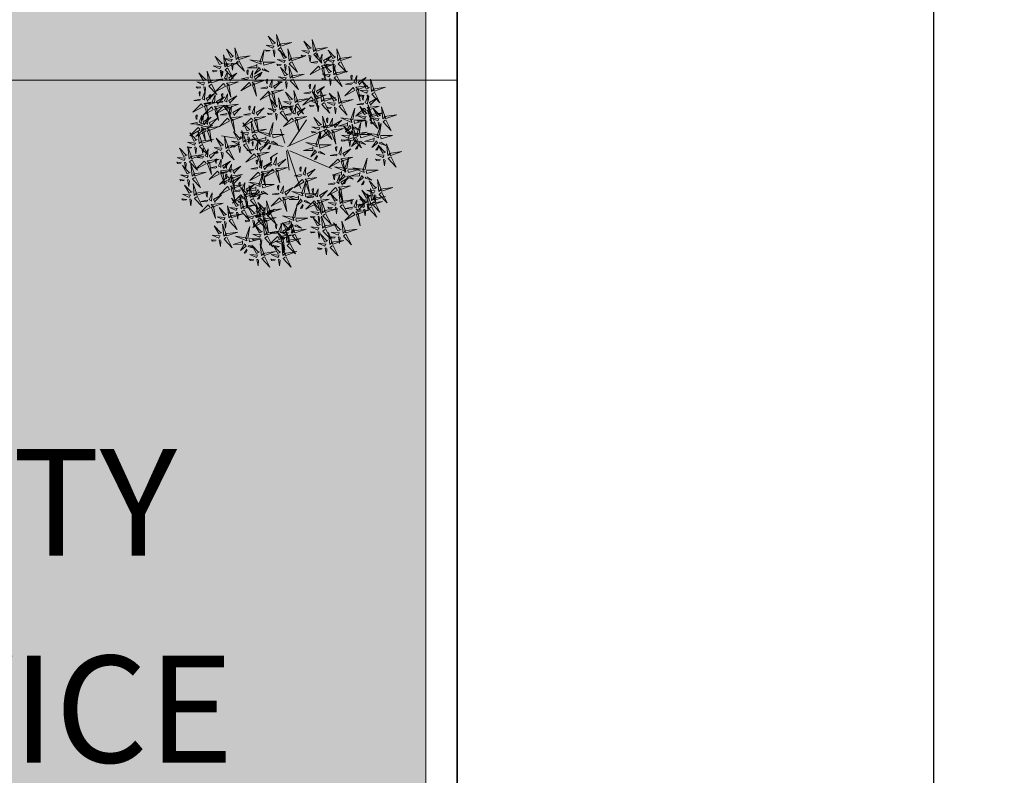
# Model space of a CAD drawing. Units: inches. Extents: x 1704 to 6393, y -157 to 1172.
# Tile 91 of 122: x 2667 to 2793, y 783 to 880. Entities that reach past the tile are written whole.
import ezdxf

# ---------------------------------------------------------------- set-up
doc = ezdxf.new("R2010")
doc.units = ezdxf.units.IN
doc.header["$MEASUREMENT"] = 0
for name, color, linetype, lineweight in [('A-ANNO-DIMS', 7, 'Continuous', 13), ('A-AREA-IDEN', 7, 'Continuous', 18), ('C-PROP', 7, 'Continuous', 35), ('L-HRDS', 8, 'Continuous', 18), ('L-shrub', 74, 'Continuous', 18), ('L-tree', 102, 'Continuous', 18)]:
    doc.layers.add(name, color=color, linetype=linetype, lineweight=lineweight)
doc.layers.add('L-HRDS-PATT', color=9, linetype='Continuous', lineweight=13, true_color=0xc5c1ba)
doc.styles.get("Standard").update_dxf_attribs({"font": 'arial.ttf'})
doc.dimstyles.get("Standard").update_dxf_attribs({"dimtxt": 6, "dimasz": 2, "dimexe": 0.18, "dimexo": 0.0625, "dimgap": 0.09, "dimtad": 0, "dimtih": 1, "dimtoh": 1, "dimdec": 1, "dimzin": 0, "dimdsep": 46, "dimlunit": 3, "dimtxsty": 'Standard', "dimblk": 'ARCHTICK', "dimcen": 0.09, "dimadec": 0, "dimazin": 0, "dimtfac": 1, "dimtdec": 1, "dimtofl": 0, "dimtmove": 0, "dimatfit": 3, "dimfxl": 1, "dimtolj": 1, "dimtzin": 0, "dimarcsym": 0})

# ---------------------------------------------------------------- blocks, each defined once
blk = doc.blocks.new('bamboo')
blk.add_line((390, 162), (546, 218))
at = {"layer": 'L-shrub'}
for p, q in [((-12, 40), (-247, 564)), ((43, 73), (278, 631)), ((-24, 62), (-370, 296)), ((32, 40), (390, 162)), ((-57, 6), (-247, -50)), ((43, 28), (301, 62)), ((-12, -16), (-113, -440)), ((77, -94), (122, -173)), ((-471, -139), (-761, -217)), ((-124, -653), (-158, -842))]:
    blk.add_line(p, q, dxfattribs=at)
for points in [[(-388, 1357), (-437, 1504), (-414, 1335), (-388, 1357)], [(104, 1425), (54, 1572), (78, 1403), (104, 1425)], [(119, 1423), (261, 1497), (148, 1389), (127, 1415)], [(582, 1302), (532, 1450), (556, 1281), (582, 1302)], [(-756, 1207), (-806, 1354), (-782, 1185), (-756, 1207)], [(-412, 1351), (-384, 1316), (-544, 1300), (-421, 1344)], [(-415, 1179), (-464, 1327), (-441, 1158), (-415, 1179)], [(-372, 1355), (-230, 1429), (-344, 1320), (-365, 1346)], [(-161, 1285), (-160, 1445), (-117, 1294), (-150, 1287)], [(-71, 1292), (-28, 1359), (-55, 1273), (-69, 1281)], [(79, 1419), (108, 1385), (-52, 1368), (71, 1412)], [(58, 1358), (77, 1316), (-31, 1255), (65, 1349)], [(103, 1337), (93, 1227), (133, 1319), (110, 1329)], [(168, 1347), (246, 1339), (158, 1324), (159, 1340)], [(597, 1300), (739, 1374), (626, 1266), (604, 1292)], [(704, 1207), (655, 1354), (679, 1185), (704, 1207)], [(-781, 1201), (-752, 1166), (-913, 1150), (-789, 1194)], [(-741, 1205), (-599, 1279), (-712, 1170), (-734, 1196)], [(-562, 1158), (-603, 1137), (-666, 1245), (-570, 1151)], [(-500, 1137), (-534, 1108), (-554, 1268), (-507, 1146)], [(-434, 1290), (-414, 1248), (-523, 1187), (-427, 1281)], [(-388, 1269), (-399, 1159), (-358, 1250), (-381, 1261)], [(-399, 1178), (-257, 1251), (-371, 1143), (-392, 1169)], [(-330, 1216), (-336, 1153), (-319, 1167), (-323, 1207)], [(-324, 1279), (-245, 1271), (-334, 1256), (-332, 1272)], [(-169, 1272), (-323, 1296), (-162, 1239), (-169, 1272)], [(-176, 1248), (-132, 1257), (-192, 1107), (-173, 1237)], [(-131, 1200), (-85, 1198), (-82, 1073), (-120, 1202)], [(-92, 1231), (0, 1171), (-62, 1249), (-81, 1233)], [(-18, 1258), (35, 1223), (30, 1245), (-7, 1260)], [(162, 1284), (156, 1221), (173, 1235), (169, 1276)], [(304, 1094), (304, 1254), (347, 1103), (314, 1096)], [(557, 1296), (586, 1262), (425, 1246), (549, 1289)], [(536, 1235), (555, 1193), (446, 1133), (543, 1226)], [(680, 1201), (709, 1166), (548, 1150), (671, 1194)], [(581, 1215), (571, 1105), (611, 1196), (588, 1206)], [(646, 1224), (724, 1217), (635, 1202), (637, 1217)], [(720, 1205), (862, 1279), (749, 1170), (727, 1196)], [(773, 1166), (723, 1313), (747, 1144), (773, 1166)], [(788, 1164), (930, 1238), (817, 1130), (796, 1155)], [(-835, 1008), (-876, 987), (-939, 1095), (-843, 1001)], [(-802, 1140), (-783, 1098), (-892, 1037), (-795, 1131)], [(-773, 987), (-807, 958), (-827, 1118), (-780, 996)], [(-757, 1119), (-767, 1009), (-727, 1100), (-750, 1111)], [(-698, 1066), (-704, 1003), (-687, 1017), (-691, 1057)], [(-692, 1129), (-614, 1121), (-703, 1106), (-701, 1122)], [(-633, 1052), (-696, 1057), (-682, 1040), (-642, 1045)], [(-581, 1112), (-692, 1120), (-599, 1081), (-590, 1104)], [(-570, 1048), (-576, 969), (-593, 1057), (-578, 1056)], [(-439, 1174), (-411, 1139), (-571, 1123), (-448, 1167)], [(-461, 1112), (-441, 1071), (-550, 1010), (-454, 1104)], [(-495, 1097), (-419, 957), (-529, 1068), (-504, 1090)], [(-494, 1113), (-347, 1165), (-516, 1138), (-494, 1113)], [(-415, 1092), (-426, 982), (-386, 1073), (-408, 1083)], [(-365, 930), (-365, 1090), (-322, 940), (-355, 933)], [(-351, 1102), (-272, 1094), (-361, 1079), (-360, 1095)], [(-156, 961), (-205, 1109), (-182, 940), (-156, 961)], [(-174, 1012), (-174, 1172), (-131, 1021), (-163, 1015)], [(-85, 1020), (-41, 1086), (-69, 1000), (-82, 1009)], [(295, 1081), (141, 1106), (302, 1048), (295, 1081)], [(289, 1057), (332, 1066), (272, 916), (291, 1046)], [(372, 1040), (465, 980), (402, 1058), (383, 1042)], [(393, 1102), (437, 1168), (409, 1082), (396, 1091)], [(446, 1067), (499, 1033), (495, 1054), (457, 1069)], [(658, 1140), (678, 1098), (569, 1037), (665, 1131)], [(748, 1160), (777, 1126), (617, 1109), (740, 1153)], [(640, 1161), (634, 1099), (651, 1113), (647, 1153)], [(727, 1099), (746, 1057), (638, 996), (734, 1090)], [(704, 1119), (694, 1009), (734, 1100), (711, 1111)], [(831, 1008), (789, 987), (726, 1095), (822, 1001)], [(762, 1066), (756, 1003), (774, 1017), (770, 1057)], [(768, 1129), (847, 1121), (758, 1106), (760, 1122)], [(772, 1078), (762, 968), (802, 1060), (779, 1070)], [(837, 1088), (915, 1080), (827, 1065), (828, 1081)], [(892, 987), (859, 958), (839, 1118), (885, 996)], [(-854, 962), (-965, 970), (-872, 931), (-863, 954)], [(-768, 947), (-692, 807), (-802, 918), (-777, 940)], [(-767, 963), (-621, 1015), (-789, 988), (-767, 963)], [(-374, 917), (-528, 942), (-367, 884), (-374, 917)], [(-357, 1039), (-363, 976), (-346, 990), (-350, 1030)], [(-183, 999), (-337, 1024), (-176, 966), (-183, 999)], [(-180, 955), (-152, 921), (-312, 905), (-189, 948)], [(-276, 938), (-232, 1004), (-260, 918), (-273, 927)], [(-189, 975), (-146, 984), (-206, 835), (-187, 964)], [(-145, 927), (-99, 925), (-96, 801), (-134, 929)], [(-140, 960), (2, 1033), (-112, 925), (-133, 951)], [(-106, 958), (-13, 898), (-75, 976), (-95, 960)], [(-32, 985), (21, 951), (17, 973), (-21, 987)], [(290, 849), (291, 1008), (334, 858), (301, 851)], [(333, 1009), (379, 1007), (382, 882), (344, 1011)], [(380, 856), (423, 922), (395, 837), (382, 845)], [(745, 784), (696, 931), (720, 762), (745, 784)], [(811, 962), (701, 970), (793, 931), (803, 954)], [(831, 1025), (825, 962), (842, 976), (838, 1016)], [(897, 947), (974, 807), (863, 918), (889, 940)], [(899, 963), (1045, 1015), (877, 988), (899, 963)], [(1141, 825), (1092, 972), (1115, 803), (1141, 825)], [(-1166, 757), (-1215, 904), (-1192, 735), (-1166, 757)], [(-1150, 755), (-1008, 829), (-1122, 721), (-1143, 746)], [(-975, 702), (-1024, 850), (-1001, 681), (-975, 702)], [(-906, 902), (-969, 907), (-955, 890), (-915, 895)], [(-843, 898), (-849, 819), (-866, 907), (-851, 906)], [(-593, 770), (-642, 918), (-618, 749), (-593, 770)], [(-577, 769), (-435, 842), (-548, 734), (-570, 760)], [(-380, 893), (-337, 902), (-397, 753), (-378, 882)], [(-336, 845), (-290, 844), (-287, 719), (-325, 848)], [(-297, 876), (-204, 816), (-266, 894), (-286, 879)], [(-202, 894), (-182, 853), (-291, 792), (-195, 885)], [(-200, 660), (-234, 631), (-253, 791), (-207, 669)], [(-223, 903), (-170, 869), (-174, 891), (-212, 906)], [(-156, 874), (-167, 764), (-126, 855), (-149, 865)], [(-98, 821), (-104, 758), (-86, 772), (-91, 812)], [(-92, 883), (-13, 876), (-102, 861), (-100, 876)], [(121, 803), (80, 783), (16, 890), (112, 796)], [(281, 835), (128, 860), (288, 803), (281, 835)], [(183, 783), (149, 754), (129, 914), (175, 791)], [(189, 759), (335, 811), (167, 784), (189, 759)], [(275, 811), (319, 820), (259, 671), (277, 800)], [(358, 795), (451, 734), (389, 812), (369, 797)], [(503, 776), (462, 755), (399, 863), (495, 769)], [(433, 822), (486, 787), (481, 809), (444, 824)], [(565, 756), (531, 726), (511, 886), (558, 764)], [(759, 902), (696, 907), (711, 890), (751, 895)], [(761, 782), (903, 856), (790, 748), (768, 774)], [(822, 898), (816, 819), (799, 907), (815, 906)], [(1117, 819), (1145, 785), (985, 768), (1108, 812)], [(1157, 823), (1299, 897), (1185, 789), (1164, 815)], [(1292, 647), (1242, 795), (1266, 626), (1292, 647)], [(-1190, 751), (-1162, 716), (-1322, 700), (-1199, 744)], [(-1212, 690), (-1192, 648), (-1301, 587), (-1205, 681)], [(-1166, 669), (-1177, 559), (-1136, 651), (-1159, 661)], [(-999, 696), (-971, 662), (-1131, 646), (-1008, 689)], [(-1102, 679), (-1023, 671), (-1112, 656), (-1111, 672)], [(-959, 700), (-817, 774), (-931, 666), (-952, 692)], [(-617, 765), (-588, 730), (-749, 714), (-626, 757)], [(-639, 703), (-619, 662), (-728, 601), (-632, 695)], [(-620, 538), (-669, 686), (-646, 517), (-620, 538)], [(-593, 683), (-603, 573), (-563, 664), (-586, 674)], [(-529, 693), (-450, 685), (-539, 670), (-537, 685)], [(-262, 681), (-303, 660), (-366, 768), (-270, 673)], [(-265, 566), (-314, 713), (-291, 544), (-265, 566)], [(-194, 636), (-47, 688), (-216, 661), (-194, 636)], [(49, 698), (-14, 702), (1, 686), (41, 690)], [(101, 757), (-9, 765), (83, 727), (93, 750)], [(112, 693), (106, 614), (89, 703), (105, 701)], [(187, 743), (264, 602), (153, 714), (179, 736)], [(319, 763), (365, 762), (369, 637), (330, 766)], [(432, 670), (369, 675), (383, 658), (423, 663)], [(484, 730), (373, 738), (465, 700), (475, 723)], [(495, 666), (489, 587), (472, 675), (487, 674)], [(570, 716), (646, 575), (536, 686), (561, 708)], [(571, 731), (717, 784), (549, 757), (571, 731)], [(721, 778), (750, 744), (589, 727), (712, 771)], [(699, 717), (719, 675), (610, 614), (706, 708)], [(745, 697), (734, 586), (775, 678), (752, 688)], [(809, 706), (888, 699), (799, 683), (801, 699)], [(868, 552), (819, 700), (842, 531), (868, 552)], [(1095, 758), (1115, 716), (1006, 655), (1102, 749)], [(1073, 552), (1024, 700), (1047, 531), (1073, 552)], [(1141, 737), (1130, 627), (1171, 719), (1148, 729)], [(1199, 684), (1193, 621), (1211, 636), (1206, 676)], [(1205, 747), (1284, 739), (1195, 724), (1197, 740)], [(1307, 646), (1449, 719), (1336, 611), (1314, 637)], [(-1289, 429), (-1338, 577), (-1315, 408), (-1289, 429)], [(-1122, 544), (-1163, 524), (-1226, 631), (-1130, 537)], [(-1108, 616), (-1114, 553), (-1097, 567), (-1101, 607)], [(-1060, 524), (-1094, 495), (-1113, 654), (-1067, 532)], [(-1021, 635), (-1001, 593), (-1110, 533), (-1014, 626)], [(-1054, 499), (-907, 552), (-1076, 525), (-1054, 499)], [(-975, 615), (-986, 505), (-945, 596), (-968, 606)], [(-917, 561), (-923, 499), (-906, 513), (-910, 553)], [(-911, 624), (-832, 617), (-921, 602), (-919, 617)], [(-712, 449), (-753, 428), (-816, 536), (-721, 441)], [(-644, 533), (-616, 498), (-776, 482), (-653, 526)], [(-650, 428), (-684, 399), (-704, 559), (-658, 437)], [(-604, 537), (-462, 610), (-576, 502), (-597, 528)], [(-535, 630), (-541, 567), (-523, 581), (-527, 621)], [(-289, 560), (-261, 526), (-421, 509), (-298, 553)], [(-333, 575), (-396, 580), (-381, 563), (-341, 568)], [(-281, 634), (-391, 643), (-299, 604), (-289, 627)], [(-270, 570), (-276, 492), (-293, 580), (-277, 579)], [(-249, 564), (-107, 638), (-221, 530), (-242, 555)], [(-195, 620), (-118, 480), (-229, 591), (-203, 613)], [(-38, 467), (-37, 627), (6, 476), (-27, 469)], [(52, 474), (95, 540), (68, 455), (54, 463)], [(680, 490), (639, 469), (576, 577), (672, 482)], [(742, 469), (708, 440), (689, 600), (735, 478)], [(844, 546), (872, 512), (712, 496), (835, 539)], [(803, 643), (797, 580), (815, 595), (810, 635)], [(884, 550), (1026, 624), (912, 516), (891, 542)], [(1049, 546), (1077, 512), (917, 496), (1040, 539)], [(1089, 550), (1231, 624), (1117, 516), (1096, 542)], [(1267, 642), (1296, 607), (1135, 591), (1259, 635)], [(1245, 580), (1265, 539), (1156, 478), (1253, 572)], [(1291, 560), (1281, 450), (1321, 541), (1298, 552)], [(1356, 570), (1434, 562), (1345, 547), (1347, 563)], [(-1313, 424), (-1285, 389), (-1445, 373), (-1322, 417)], [(-1273, 428), (-1131, 501), (-1245, 393), (-1266, 419)], [(-1193, 439), (-1256, 443), (-1242, 426), (-1202, 431)], [(-1141, 498), (-1251, 506), (-1159, 468), (-1150, 491)], [(-1130, 434), (-1136, 355), (-1153, 444), (-1137, 442)], [(-1055, 484), (-979, 343), (-1089, 455), (-1063, 476)], [(-731, 403), (-842, 411), (-750, 372), (-740, 395)], [(-666, 471), (-646, 430), (-755, 369), (-659, 463)], [(-644, 404), (-498, 456), (-666, 429), (-644, 404)], [(-620, 451), (-631, 341), (-590, 432), (-613, 442)], [(-562, 398), (-568, 335), (-551, 349), (-555, 389)], [(-556, 461), (-477, 453), (-566, 438), (-564, 454)], [(-311, 499), (-291, 457), (-400, 396), (-304, 490)], [(-265, 478), (-276, 368), (-235, 460), (-258, 470)], [(-207, 425), (-213, 362), (-196, 376), (-200, 416)], [(-201, 488), (-122, 480), (-211, 465), (-210, 481)], [(-46, 454), (-200, 478), (-40, 421), (-46, 454)], [(-53, 429), (-9, 439), (-69, 289), (-50, 418)], [(31, 413), (123, 352), (61, 431), (42, 415)], [(105, 440), (158, 405), (153, 427), (116, 442)], [(394, 326), (353, 305), (290, 413), (385, 319)], [(456, 306), (422, 276), (402, 436), (448, 314)], [(661, 444), (551, 452), (643, 413), (653, 436)], [(618, 276), (618, 436), (661, 285), (628, 278)], [(747, 429), (824, 289), (713, 400), (739, 422)], [(748, 445), (895, 497), (727, 470), (748, 445)], [(822, 485), (842, 443), (733, 383), (829, 476)], [(868, 465), (857, 355), (898, 446), (875, 456)], [(926, 411), (920, 349), (937, 363), (933, 403)], [(932, 474), (1011, 467), (922, 452), (924, 467)], [(1027, 485), (1047, 443), (938, 383), (1034, 476)], [(1073, 465), (1062, 355), (1103, 446), (1080, 456)], [(1131, 411), (1125, 349), (1142, 363), (1138, 403)], [(1137, 474), (1216, 467), (1127, 452), (1128, 467)], [(1349, 507), (1343, 444), (1361, 458), (1357, 498)], [(-1335, 362), (-1315, 321), (-1424, 260), (-1328, 354)], [(-1289, 342), (-1300, 232), (-1259, 323), (-1282, 333)], [(-1231, 289), (-1237, 226), (-1220, 240), (-1224, 280)], [(-1225, 352), (-1146, 344), (-1235, 329), (-1233, 345)], [(-784, 343), (-847, 348), (-832, 331), (-792, 336)], [(-721, 338), (-727, 260), (-744, 348), (-728, 347)], [(-645, 388), (-569, 248), (-679, 359), (-654, 381)], [(-606, 184), (-656, 331), (-632, 163), (-606, 184)], [(-425, 190), (-467, 169), (-530, 277), (-434, 182)], [(-364, 169), (-397, 140), (-417, 300), (-371, 178)], [(-8, 382), (38, 380), (41, 255), (2, 384)], [(374, 280), (264, 288), (356, 250), (366, 273)], [(460, 266), (537, 125), (427, 236), (452, 258)], [(462, 281), (608, 334), (440, 307), (462, 281)], [(609, 263), (455, 287), (616, 230), (609, 263)], [(609, 384), (546, 389), (561, 372), (601, 377)], [(672, 379), (666, 301), (649, 389), (665, 388)], [(707, 283), (751, 349), (723, 264), (710, 272)], [(945, 153), (946, 313), (989, 162), (956, 155)], [(1141, 143), (1092, 291), (1115, 122), (1141, 143)], [(-1166, 102), (-1215, 250), (-1192, 81), (-1166, 102)], [(-1150, 100), (-1008, 174), (-1122, 66), (-1143, 92)], [(-934, 116), (-983, 263), (-960, 94), (-934, 116)], [(-918, 114), (-776, 188), (-890, 80), (-911, 105)], [(-631, 178), (-602, 144), (-762, 128), (-639, 171)], [(-590, 182), (-449, 256), (-562, 148), (-583, 174)], [(-445, 144), (-555, 152), (-463, 113), (-453, 136)], [(-358, 145), (-211, 197), (-379, 170), (-358, 145)], [(322, 220), (259, 225), (274, 208), (314, 213)], [(385, 216), (379, 137), (362, 225), (378, 224)], [(603, 239), (646, 248), (586, 98), (605, 228)], [(647, 191), (693, 189), (696, 64), (658, 193)], [(701, 6), (667, -24), (648, 136), (694, 14)], [(686, 222), (779, 161), (716, 240), (697, 224)], [(760, 249), (813, 214), (809, 236), (771, 251)], [(937, 140), (783, 165), (943, 107), (937, 140)], [(1117, 137), (1145, 103), (985, 87), (1108, 130)], [(1035, 161), (1078, 227), (1051, 141), (1037, 150)], [(1157, 141), (1299, 215), (1185, 107), (1164, 133)], [(1264, 75), (1215, 222), (1238, 53), (1264, 75)], [(1280, 73), (1422, 147), (1308, 39), (1287, 65)], [(1442, 20), (1392, 168), (1416, -1), (1442, 20)], [(-1357, -48), (-1406, 100), (-1383, -69), (-1357, -48)], [(-1341, -50), (-1199, 24), (-1313, -84), (-1334, -58)], [(-1190, 96), (-1162, 62), (-1322, 46), (-1199, 89)], [(-1212, 35), (-1192, -7), (-1301, -67), (-1205, 26)], [(-1166, 15), (-1177, -95), (-1136, -4), (-1159, 6)], [(-1102, 24), (-1023, 17), (-1112, 2), (-1111, 17)], [(-958, 110), (-930, 76), (-1090, 59), (-967, 103)], [(-980, 49), (-960, 7), (-1069, -54), (-973, 40)], [(-934, 28), (-945, -82), (-904, 10), (-927, 20)], [(-870, 38), (-791, 30), (-880, 15), (-878, 31)], [(-652, 117), (-632, 75), (-741, 14), (-645, 108)], [(-607, 97), (-617, -13), (-577, 78), (-600, 88)], [(-511, -21), (-560, 127), (-536, -42), (-511, -21)], [(-497, 84), (-560, 89), (-545, 72), (-505, 77)], [(-548, 43), (-554, -20), (-537, -5), (-541, 35)], [(-542, 106), (-464, 99), (-552, 83), (-551, 99)], [(-495, -22), (-353, 51), (-466, -57), (-488, -31)], [(-434, 79), (-440, 1), (-457, 89), (-441, 88)], [(-359, 129), (-282, -11), (-393, 100), (-367, 122)], [(257, -69), (216, -90), (153, 18), (249, -77)], [(319, -90), (285, -119), (266, 41), (312, -81)], [(640, 26), (598, 5), (535, 113), (631, 19)], [(707, -19), (854, 34), (686, 7), (707, -19)], [(930, 116), (974, 125), (914, -24), (932, 105)], [(974, 68), (1021, 66), (1024, -58), (985, 70)], [(1095, 76), (1115, 34), (1006, -27), (1102, 67)], [(1014, 99), (1106, 39), (1044, 117), (1025, 101)], [(1158, -1), (1117, -22), (1054, 86), (1150, -9)], [(1088, 126), (1141, 92), (1136, 113), (1099, 128)], [(1240, 69), (1268, 35), (1108, 18), (1231, 62)], [(1218, 8), (1238, -34), (1129, -95), (1225, -1)], [(1141, 56), (1130, -54), (1171, 37), (1148, 47)], [(1220, -22), (1186, -51), (1167, 109), (1213, -13)], [(1199, 2), (1193, -60), (1211, -46), (1206, -6)], [(1205, 65), (1284, 58), (1195, 42), (1197, 58)], [(1226, -46), (1373, 6), (1204, -21), (1226, -46)], [(1417, 15), (1446, -20), (1286, -36), (1409, 8)], [(1457, 19), (1599, 92), (1486, -16), (1465, 10)], [(-1381, -54), (-1353, -88), (-1513, -104), (-1390, -61)], [(-1403, -115), (-1383, -157), (-1492, -217), (-1396, -124)], [(-1293, -126), (-1215, -133), (-1303, -148), (-1302, -133)], [(-1144, -283), (-1143, -123), (-1100, -274), (-1133, -281)], [(-1108, -39), (-1114, -101), (-1097, -87), (-1101, -47)], [(-780, -124), (-822, -145), (-885, -37), (-789, -131)], [(-876, -25), (-882, -88), (-865, -74), (-869, -33)], [(-719, -144), (-752, -174), (-772, -14), (-726, -136)], [(-712, -169), (-566, -116), (-734, -143), (-712, -169)], [(-535, -26), (-507, -61), (-667, -77), (-544, -33)], [(-557, -88), (-537, -129), (-646, -190), (-550, -96)], [(-511, -108), (-522, -218), (-481, -127), (-504, -117)], [(-447, -98), (-368, -106), (-457, -121), (-455, -105)], [(-174, -160), (-174, -1), (-131, -151), (-163, -158)], [(-85, -153), (-41, -87), (-69, -173), (-82, -164)], [(238, -116), (128, -107), (220, -146), (229, -123)], [(324, -130), (400, -270), (290, -159), (315, -137)], [(325, -114), (472, -62), (303, -89), (325, -114)], [(568, -80), (505, -75), (520, -92), (560, -87)], [(620, -20), (510, -12), (602, -50), (612, -27)], [(631, -84), (625, -163), (608, -75), (624, -76)], [(706, -34), (783, -175), (672, -64), (698, -42)], [(868, -184), (819, -37), (842, -206), (868, -184)], [(884, -186), (1026, -112), (912, -220), (891, -194)], [(988, -240), (954, -269), (935, -109), (981, -231)], [(1087, -107), (1024, -102), (1038, -119), (1078, -114)], [(1139, -47), (1029, -39), (1121, -78), (1130, -55)], [(1169, -225), (1119, -78), (1143, -247), (1169, -225)], [(1150, -112), (1144, -190), (1127, -102), (1143, -103)], [(1225, -62), (1301, -202), (1191, -91), (1217, -69)], [(1264, -13), (1253, -123), (1294, -31), (1271, -21)], [(1396, -47), (1415, -88), (1306, -149), (1403, -55)], [(1322, -66), (1316, -129), (1333, -114), (1329, -74)], [(1328, -3), (1407, -10), (1318, -26), (1320, -10)], [(1442, -266), (1392, -119), (1416, -287), (1442, -266)], [(1441, -67), (1431, -177), (1471, -86), (1448, -76)], [(1500, -120), (1494, -183), (1511, -169), (1507, -129)], [(1506, -57), (1584, -65), (1496, -80), (1497, -65)], [(-1358, -135), (-1368, -245), (-1328, -154), (-1350, -144)], [(-1299, -188), (-1305, -251), (-1288, -237), (-1292, -197)], [(-1054, -276), (-1011, -210), (-1038, -295), (-1052, -287)], [(-852, -230), (-915, -225), (-900, -242), (-860, -237)], [(-800, -170), (-910, -162), (-818, -200), (-808, -177)], [(-789, -234), (-795, -313), (-812, -225), (-796, -226)], [(-714, -184), (-637, -325), (-748, -214), (-722, -192)], [(-453, -161), (-459, -224), (-441, -210), (-446, -170)], [(-364, -376), (-397, -405), (-417, -246), (-371, -368)], [(-183, -174), (-337, -149), (-176, -206), (-183, -174)], [(-197, -389), (-246, -241), (-222, -410), (-197, -389)], [(-189, -198), (-146, -189), (-206, -338), (-187, -209)], [(-145, -246), (-99, -247), (-96, -372), (-134, -243)], [(-106, -215), (-13, -275), (-75, -197), (-95, -212)], [(52, -315), (11, -336), (-52, -228), (44, -322)], [(-32, -187), (21, -222), (17, -200), (-21, -185)], [(114, -335), (80, -364), (61, -205), (107, -327)], [(186, -175), (123, -170), (137, -187), (177, -182)], [(298, -260), (257, -281), (194, -173), (290, -268)], [(249, -180), (243, -258), (226, -170), (242, -171)], [(360, -281), (326, -310), (307, -150), (353, -272)], [(366, -305), (513, -253), (344, -280), (366, -305)], [(495, -297), (495, -137), (538, -288), (506, -295)], [(584, -289), (628, -223), (600, -309), (587, -300)], [(844, -190), (872, -224), (712, -241), (835, -197)], [(822, -251), (842, -293), (733, -354), (829, -260)], [(907, -266), (797, -257), (889, -296), (898, -273)], [(926, -219), (885, -240), (822, -132), (918, -227)], [(923, -321), (874, -173), (897, -342), (923, -321)], [(932, -262), (1011, -270), (922, -285), (924, -269)], [(939, -322), (1081, -249), (967, -357), (946, -331)], [(994, -264), (1141, -212), (972, -239), (994, -264)], [(1144, -231), (1173, -265), (1013, -282), (1136, -238)], [(1184, -227), (1326, -153), (1213, -261), (1191, -235)], [(1457, -268), (1599, -194), (1486, -302), (1465, -276)], [(-1152, -296), (-1306, -272), (-1145, -329), (-1152, -296)], [(-1159, -321), (-1115, -311), (-1175, -461), (-1156, -331)], [(-1114, -368), (-1068, -370), (-1065, -495), (-1103, -366)], [(-1075, -337), (-983, -398), (-1045, -319), (-1064, -335)], [(-903, -383), (-944, -404), (-1007, -296), (-912, -390)], [(-1001, -310), (-948, -345), (-953, -323), (-990, -308)], [(-841, -404), (-875, -433), (-895, -273), (-849, -395)], [(-835, -428), (-689, -375), (-857, -402), (-835, -428)], [(-445, -402), (-555, -394), (-463, -432), (-453, -409)], [(-425, -356), (-467, -376), (-530, -269), (-434, -363)], [(-358, -400), (-211, -348), (-379, -375), (-358, -400)], [(-221, -394), (-193, -429), (-353, -445), (-230, -402)], [(-181, -390), (-39, -317), (-152, -425), (-174, -399)], [(-74, -512), (-123, -364), (-100, -533), (-74, -512)], [(33, -361), (-77, -353), (15, -391), (25, -368)], [(119, -375), (196, -516), (85, -404), (111, -383)], [(120, -360), (267, -307), (99, -334), (120, -360)], [(227, -366), (164, -361), (178, -378), (218, -373)], [(279, -306), (169, -298), (261, -337), (270, -314)], [(290, -371), (284, -449), (267, -361), (283, -362)], [(365, -321), (441, -461), (331, -350), (356, -328)], [(486, -310), (332, -285), (493, -343), (486, -310)], [(480, -334), (523, -325), (463, -474), (482, -345)], [(524, -382), (570, -384), (573, -508), (535, -380)], [(563, -351), (656, -411), (594, -333), (574, -349)], [(660, -513), (626, -542), (607, -382), (653, -504)], [(663, -416), (614, -269), (638, -437), (663, -416)], [(637, -324), (690, -358), (686, -336), (648, -322)], [(679, -418), (821, -344), (708, -452), (686, -426)], [(814, -539), (764, -391), (788, -560), (814, -539)], [(899, -326), (927, -361), (767, -377), (890, -333)], [(877, -388), (897, -429), (788, -490), (884, -396)], [(855, -325), (792, -320), (806, -337), (846, -332)], [(868, -272), (857, -382), (898, -290), (875, -280)], [(918, -330), (912, -408), (895, -320), (911, -321)], [(926, -325), (920, -388), (937, -374), (933, -333)], [(993, -280), (1069, -420), (959, -309), (984, -287)], [(1123, -292), (1142, -334), (1033, -395), (1130, -301)], [(1168, -312), (1158, -423), (1198, -331), (1175, -321)], [(1218, -474), (1219, -314), (1262, -465), (1229, -472)], [(1227, -366), (1221, -429), (1238, -414), (1234, -374)], [(1233, -303), (1311, -310), (1223, -326), (1224, -310)], [(1417, -272), (1446, -306), (1286, -322), (1409, -279)], [(1396, -333), (1415, -375), (1306, -436), (1403, -342)], [(1441, -353), (1431, -463), (1471, -372), (1448, -362)], [(1506, -344), (1584, -351), (1496, -367), (1497, -351)], [(-1180, -607), (-1229, -459), (-1205, -628), (-1180, -607)], [(-975, -489), (-1038, -484), (-1023, -501), (-983, -496)], [(-923, -429), (-1033, -421), (-941, -459), (-931, -436)], [(-912, -493), (-918, -572), (-935, -484), (-919, -485)], [(-837, -444), (-760, -584), (-870, -473), (-845, -451)], [(-497, -461), (-560, -457), (-545, -474), (-505, -469)], [(-434, -466), (-440, -545), (-457, -456), (-441, -458)], [(-359, -416), (-282, -557), (-393, -445), (-367, -424)], [(-243, -456), (-223, -497), (-332, -558), (-236, -464)], [(-98, -517), (-70, -552), (-230, -568), (-107, -524)], [(-197, -476), (-208, -586), (-167, -495), (-190, -485)], [(-133, -466), (-54, -474), (-143, -489), (-141, -474)], [(-19, -420), (-82, -416), (-67, -433), (-27, -428)], [(-58, -513), (84, -440), (-30, -548), (-51, -522)], [(44, -425), (38, -504), (21, -415), (37, -417)], [(599, -492), (557, -513), (494, -405), (590, -499)], [(639, -422), (668, -456), (507, -472), (631, -429)], [(617, -483), (637, -525), (528, -586), (625, -492)], [(666, -537), (813, -484), (645, -511), (666, -537)], [(663, -503), (653, -613), (693, -522), (670, -512)], [(727, -494), (806, -501), (717, -517), (719, -501)], [(829, -540), (971, -467), (858, -575), (836, -549)], [(922, -408), (912, -518), (952, -427), (930, -417)], [(981, -461), (975, -524), (992, -510), (988, -470)], [(987, -398), (1065, -406), (977, -421), (978, -405)], [(1210, -487), (1056, -463), (1216, -520), (1210, -487)], [(1203, -511), (1247, -502), (1187, -652), (1206, -522)], [(1287, -528), (1379, -588), (1317, -510), (1298, -526)], [(1308, -467), (1351, -400), (1324, -486), (1310, -478)], [(1361, -501), (1414, -536), (1409, -514), (1372, -499)], [(1500, -407), (1494, -470), (1511, -455), (1507, -415)], [(-1204, -613), (-1176, -647), (-1336, -663), (-1213, -620)], [(-1164, -609), (-1022, -535), (-1135, -643), (-1157, -617)], [(-1084, -757), (-1133, -609), (-1110, -778), (-1084, -757)], [(-890, -724), (-931, -745), (-994, -637), (-898, -731)], [(-828, -744), (-862, -774), (-881, -614), (-835, -736)], [(-589, -724), (-630, -745), (-693, -637), (-598, -731)], [(-527, -744), (-561, -774), (-581, -614), (-535, -736)], [(-425, -669), (-467, -690), (-530, -582), (-434, -677)], [(-364, -690), (-397, -719), (-417, -559), (-371, -681)], [(-120, -579), (-100, -620), (-209, -681), (-113, -587)], [(-139, -529), (-145, -592), (-127, -578), (-132, -538)], [(-74, -599), (-85, -709), (-44, -618), (-67, -607)], [(8, -743), (-41, -596), (-18, -765), (8, -743)], [(-16, -652), (-22, -715), (-5, -701), (-9, -661)], [(-10, -589), (69, -597), (-20, -612), (-18, -596)], [(353, -669), (312, -690), (249, -582), (344, -677)], [(415, -690), (381, -719), (361, -559), (407, -681)], [(489, -669), (448, -690), (385, -582), (481, -677)], [(527, -598), (464, -593), (479, -610), (519, -605)], [(579, -538), (469, -530), (561, -569), (571, -546)], [(551, -690), (517, -719), (498, -559), (544, -681)], [(590, -602), (584, -681), (567, -593), (583, -594)], [(665, -553), (742, -693), (631, -582), (657, -560)], [(789, -544), (818, -579), (658, -595), (781, -552)], [(768, -606), (787, -647), (678, -708), (775, -614)], [(721, -557), (715, -620), (733, -605), (729, -565)], [(813, -626), (803, -736), (843, -645), (820, -635)], [(878, -616), (956, -624), (868, -639), (869, -624)], [(937, -703), (887, -555), (911, -724), (937, -703)], [(952, -704), (1094, -630), (981, -739), (959, -713)], [(1182, -771), (1133, -623), (1156, -792), (1182, -771)], [(1248, -559), (1294, -561), (1297, -686), (1258, -557)], [(-1226, -674), (-1206, -716), (-1315, -776), (-1219, -683)], [(-1108, -763), (-1080, -797), (-1240, -813), (-1117, -770)], [(-1180, -694), (-1191, -804), (-1150, -713), (-1173, -703)], [(-1122, -748), (-1128, -810), (-1110, -796), (-1115, -756)], [(-1116, -685), (-1037, -692), (-1126, -707), (-1124, -692)], [(-1068, -759), (-926, -685), (-1040, -793), (-1061, -767)], [(-909, -770), (-1019, -762), (-927, -800), (-917, -777)], [(-823, -784), (-746, -925), (-857, -814), (-831, -792)], [(-822, -769), (-675, -716), (-844, -743), (-822, -769)], [(-609, -770), (-719, -762), (-627, -800), (-617, -777)], [(-514, -908), (-548, -937), (-567, -777), (-521, -900)], [(-497, -775), (-560, -770), (-545, -787), (-505, -782)], [(-523, -784), (-446, -925), (-556, -814), (-531, -792)], [(-445, -715), (-555, -707), (-463, -746), (-453, -723)], [(-521, -769), (-375, -716), (-543, -743), (-521, -769)], [(-434, -780), (-440, -858), (-457, -770), (-441, -771)], [(-359, -730), (-282, -870), (-393, -759), (-367, -737)], [(-358, -714), (-211, -662), (-379, -689), (-358, -714)], [(-16, -749), (12, -783), (-148, -800), (-25, -756)], [(24, -745), (166, -671), (52, -779), (31, -754)], [(285, -806), (243, -826), (180, -719), (276, -813)], [(281, -775), (218, -770), (233, -787), (273, -782)], [(333, -715), (223, -707), (315, -746), (325, -723)], [(346, -826), (312, -855), (293, -696), (339, -818)], [(344, -780), (338, -858), (321, -770), (337, -771)], [(418, -775), (355, -770), (369, -787), (409, -782)], [(470, -715), (360, -707), (452, -746), (462, -723)], [(419, -730), (496, -870), (386, -759), (411, -737)], [(421, -714), (567, -662), (399, -689), (421, -714)], [(481, -780), (475, -858), (458, -770), (474, -771)], [(556, -730), (632, -870), (522, -759), (548, -737)], [(557, -714), (704, -662), (535, -689), (557, -714)], [(912, -708), (941, -743), (780, -759), (904, -715)], [(890, -769), (910, -811), (801, -872), (898, -778)], [(872, -679), (866, -742), (883, -728), (879, -688)], [(936, -790), (926, -900), (966, -809), (943, -798)], [(1001, -780), (1079, -788), (990, -803), (992, -787)], [(1158, -776), (1186, -811), (1026, -827), (1149, -783)], [(1198, -772), (1340, -699), (1226, -807), (1205, -781)], [(-1130, -824), (-1110, -866), (-1219, -926), (-1123, -833)], [(-1084, -844), (-1095, -954), (-1055, -863), (-1077, -853)], [(-1026, -898), (-1032, -960), (-1015, -946), (-1019, -906)], [(-1020, -835), (-941, -842), (-1030, -857), (-1029, -842)], [(-961, -829), (-1024, -825), (-1009, -842), (-969, -837)], [(-898, -834), (-904, -913), (-921, -825), (-905, -826)], [(-866, -975), (-915, -828), (-891, -997), (-866, -975)], [(-850, -977), (-708, -903), (-821, -1011), (-843, -985)], [(-661, -829), (-724, -825), (-709, -842), (-669, -837)], [(-576, -888), (-617, -908), (-680, -801), (-584, -895)], [(-598, -834), (-604, -913), (-621, -825), (-605, -826)], [(-555, -1044), (-589, -1074), (-608, -914), (-562, -1036)], [(-508, -932), (-361, -880), (-530, -907), (-508, -932)], [(-289, -983), (-330, -1004), (-393, -896), (-297, -990)], [(-227, -1004), (-261, -1033), (-280, -873), (-234, -995)], [(-38, -810), (-18, -852), (-127, -913), (-31, -819)], [(8, -831), (-3, -941), (38, -849), (15, -839)], [(148, -983), (107, -1004), (44, -896), (140, -990)], [(66, -884), (60, -947), (77, -933), (73, -893)], [(72, -821), (151, -829), (62, -844), (64, -828)], [(213, -911), (150, -907), (165, -924), (205, -919)], [(265, -852), (155, -844), (247, -882), (257, -859)], [(210, -1004), (176, -1033), (156, -873), (203, -995)], [(276, -916), (270, -995), (253, -906), (269, -908)], [(351, -866), (428, -1007), (317, -895), (343, -873)], [(352, -850), (499, -798), (331, -825), (352, -850)], [(735, -928), (694, -949), (631, -841), (727, -936)], [(797, -949), (763, -978), (743, -818), (790, -941)], [(803, -973), (950, -921), (781, -948), (803, -973)], [(995, -843), (989, -906), (1006, -892), (1002, -852)], [(1136, -838), (1156, -879), (1047, -940), (1143, -846)], [(1182, -858), (1171, -968), (1212, -877), (1189, -867)], [(1240, -911), (1234, -974), (1251, -960), (1247, -920)], [(1246, -848), (1325, -856), (1236, -871), (1238, -855)], [(-890, -981), (-862, -1015), (-1022, -1032), (-899, -988)], [(-912, -1042), (-892, -1084), (-1001, -1145), (-905, -1051)], [(-802, -1053), (-723, -1060), (-812, -1076), (-810, -1060)], [(-617, -1024), (-658, -1045), (-721, -937), (-625, -1031)], [(-647, -993), (-710, -988), (-695, -1005), (-655, -1000)], [(-595, -934), (-705, -925), (-613, -964), (-603, -941)], [(-584, -998), (-590, -1077), (-607, -988), (-591, -989)], [(-549, -1069), (-402, -1016), (-570, -1043), (-549, -1069)], [(-509, -948), (-432, -1088), (-543, -977), (-517, -955)], [(-308, -1029), (-418, -1021), (-326, -1059), (-317, -1036)], [(-303, -1065), (-344, -1086), (-407, -978), (-311, -1072)], [(-241, -1085), (-275, -1114), (-294, -955), (-248, -1077)], [(-222, -1043), (-146, -1184), (-256, -1073), (-231, -1051)], [(-221, -1028), (-74, -975), (-243, -1002), (-221, -1028)], [(-60, -1098), (-109, -950), (-86, -1119), (-60, -1098)], [(-44, -1099), (98, -1026), (-16, -1134), (-37, -1108)], [(129, -1029), (18, -1021), (111, -1059), (120, -1036)], [(215, -1043), (291, -1184), (181, -1073), (206, -1051)], [(216, -1028), (362, -975), (194, -1002), (216, -1028)], [(377, -1193), (327, -1046), (351, -1215), (377, -1193)], [(636, -1166), (587, -1019), (610, -1187), (636, -1166)], [(664, -1034), (601, -1029), (615, -1046), (655, -1041)], [(716, -975), (605, -966), (698, -1005), (707, -982)], [(727, -1039), (721, -1117), (704, -1029), (719, -1030)], [(802, -989), (878, -1129), (768, -1018), (793, -996)], [(-866, -1062), (-877, -1173), (-836, -1081), (-859, -1071)], [(-808, -1116), (-814, -1179), (-796, -1164), (-801, -1124)], [(-688, -1129), (-751, -1125), (-736, -1142), (-696, -1137)], [(-636, -1070), (-746, -1062), (-654, -1100), (-644, -1077)], [(-625, -1134), (-631, -1213), (-648, -1125), (-632, -1126)], [(-550, -1084), (-473, -1225), (-584, -1114), (-558, -1092)], [(-374, -1170), (-437, -1166), (-422, -1183), (-382, -1178)], [(-322, -1111), (-432, -1103), (-340, -1141), (-330, -1118)], [(-360, -1089), (-423, -1084), (-409, -1101), (-369, -1096)], [(-311, -1175), (-317, -1254), (-334, -1165), (-318, -1167)], [(-297, -1093), (-303, -1172), (-320, -1084), (-305, -1085)], [(-236, -1125), (-159, -1266), (-270, -1154), (-244, -1133)], [(-235, -1110), (-88, -1057), (-256, -1084), (-235, -1110)], [(-84, -1104), (-56, -1138), (-216, -1154), (-93, -1111)], [(-106, -1165), (-86, -1206), (-195, -1267), (-99, -1174)], [(-61, -1185), (-71, -1295), (-31, -1204), (-53, -1194)], [(4, -1176), (83, -1183), (-6, -1198), (-5, -1183)], [(77, -1089), (14, -1084), (28, -1101), (68, -1096)], [(145, -1234), (95, -1087), (119, -1256), (145, -1234)], [(140, -1093), (134, -1172), (117, -1084), (132, -1085)], [(160, -1236), (302, -1162), (189, -1270), (168, -1244)], [(393, -1195), (534, -1121), (421, -1229), (400, -1204)], [(612, -1172), (640, -1206), (480, -1222), (603, -1179)], [(652, -1168), (794, -1094), (680, -1202), (659, -1176)], [(120, -1240), (149, -1274), (-11, -1291), (112, -1247)], [(-2, -1238), (-8, -1301), (9, -1287), (5, -1247)], [(99, -1301), (118, -1343), (9, -1404), (106, -1310)], [(209, -1312), (287, -1320), (199, -1335), (200, -1319)], [(352, -1199), (381, -1233), (221, -1250), (344, -1206)], [(331, -1260), (351, -1302), (242, -1363), (338, -1269)], [(376, -1281), (366, -1391), (406, -1299), (383, -1289)], [(441, -1271), (519, -1279), (431, -1294), (432, -1278)], [(590, -1233), (610, -1275), (501, -1336), (597, -1242)], [(636, -1253), (625, -1363), (666, -1272), (643, -1262)], [(694, -1307), (688, -1370), (705, -1355), (701, -1315)], [(700, -1244), (779, -1251), (690, -1267), (692, -1251)], [(144, -1322), (134, -1432), (174, -1340), (151, -1330)], [(203, -1375), (197, -1438), (214, -1424), (210, -1383)], [(435, -1334), (429, -1397), (446, -1383), (442, -1343)]]:
    blk.add_lwpolyline(points, dxfattribs=at)
blk = doc.blocks.new('_ArchTick')
at = {"color": 0, "linetype": 'ByBlock', "const_width": 0.15}
blk.add_lwpolyline([(-0.5, -0.5), (0.5, 0.5)], dxfattribs=at)
blk = doc.blocks.new('*D91')
at = {"layer": 'A-ANNO-DIMS', "color": 0, "lineweight": -2, "transparency": 16777216}
for p, q in [((2723.41, 1033.21), (2784.53, 1033.21)), ((2784.35, 1033.21), (2784.35, 517.87)), ((2784.35, -3.79), (2784.35, 511.56)), ((2723.41, -3.79), (2784.53, -3.79))]:
    blk.add_line(p, q, dxfattribs=at)
at = {"layer": 'Defpoints', "color": 0, "lineweight": -3, "transparency": 16777216}
for p in [(2723.35, 1033.21), (2784.35, 1033.21), (2723.35, -3.79)]:
    blk.add_point(p, dxfattribs=at)
at = {"layer": 'A-ANNO-DIMS', "color": 0, "lineweight": -2, "transparency": 16777216, "xscale": 2, "yscale": 2, "zscale": 2}
for p, rotation in [((2784.35, 1033.21), 90), ((2784.35, -3.79), 270)]:
    blk.add_blockref('_ArchTick', p, dxfattribs=dict(at, rotation=rotation))
at = {"layer": 'A-ANNO-DIMS', "color": 0, "transparency": 16777216, "insert": (2784.35, 514.71), "char_height": 6, "attachment_point": 5}
blk.add_mtext('\\A1;1037', dxfattribs=at)

msp = doc.modelspace()

# ---------------------------------------------------------------- hatches: boundary and pattern name
at = {"layer": 'L-HRDS-PATT', "transparency": 33554661}
h = msp.add_hatch(color=256, dxfattribs=at)
h.dxf.hatch_style = 1
h.paths.add_polyline_path([(2719.349, 1033.213), (2664.349, 1033.213), (2664.349, 895.213), (2719.349, 895.213)])
h.paths.add_polyline_path([(2719.349, 895.213), (2664.349, 895.213), (2605.349, 895.213), (2605.349, 872.213), (2719.349, 872.213)])
h.paths.add_polyline_path([(2719.349, 872.213), (2605.349, 872.213), (2605.349, 854.213), (2601.349, 854.213, -0.1210664), (2618.034, 850.113), (2618.05, 850.14), (2619.349, 849.39), (2601.349, 818.213), (2605.349, 818.213), (2605.349, 794.213), (2605.349, 754.213), (2631.349, 754.213), (2631.349, 716.213), (2719.349, 716.213)])

# ---------------------------------------------------------------- linework, layer by layer
at = {"layer": 'C-PROP'}
msp.add_line((2723.349, -3.787), (2723.349, 1033.213), dxfattribs=at)
at = {"layer": 'L-HRDS'}
for p, q in [((2719.349, 5.658), (2719.349, 1033.213)), ((2605.349, 872.213), (2723.349, 872.213))]:
    msp.add_line(p, q, dxfattribs=at)

# ---------------------------------------------------------------- block references
at = {"layer": 'L-tree', "xscale": 0.0095734028514679, "yscale": 0.0095734028514679, "zscale": 0.0095734028514679, "rotation": 269.9999999999999}
msp.add_blockref('bamboo', (2701.239, 863.599), dxfattribs=at)

# ---------------------------------------------------------------- texts
at = {"layer": 'A-AREA-IDEN'}
for s, p in [('UTILITY', (2620.76, 811.34)), ('SERVICE', (2621.754, 784.847))]:
    msp.add_text(s, height=13.6672, dxfattribs=at).set_placement(p)

# ---------------------------------------------------------------- dimensions: what is measured, and where the dimension line sits
at = {"layer": 'A-ANNO-DIMS'}
dim = msp.add_linear_dim(base=(2784.349, 1033.213), p1=(2723.349, -3.787), p2=(2723.349, 1033.213), angle=90, dimstyle='Standard', override={"dimdec": 0, "dimlfac": 1, "dimrnd": 0, "dimzin": 0, "dimdsep": 46, "dimlunit": 2}, dxfattribs=at)
dim.commit()
dim.dimension.update_dxf_attribs({"geometry": '*D91', "text_midpoint": (2784.349, 514.713)})

doc.saveas('drawing.dxf')
